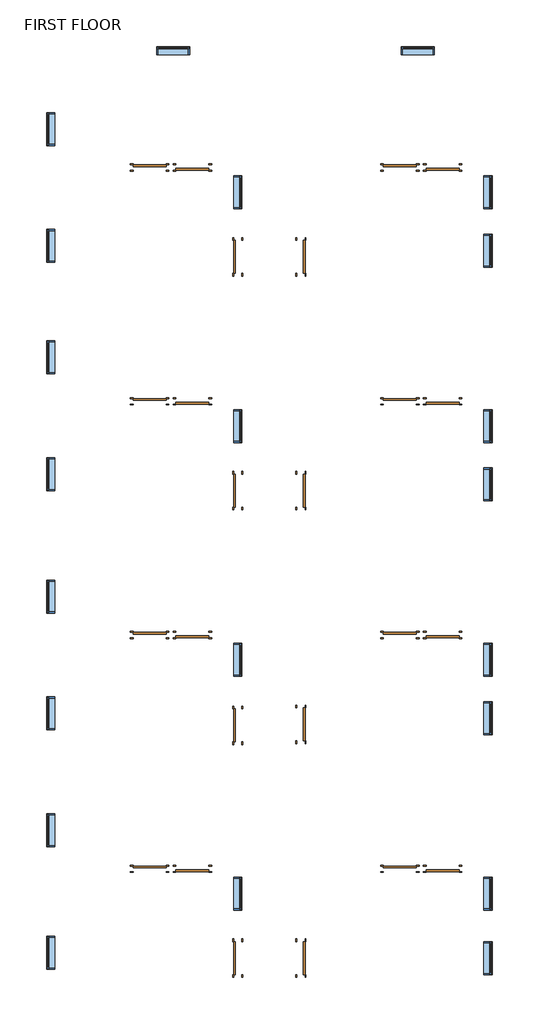
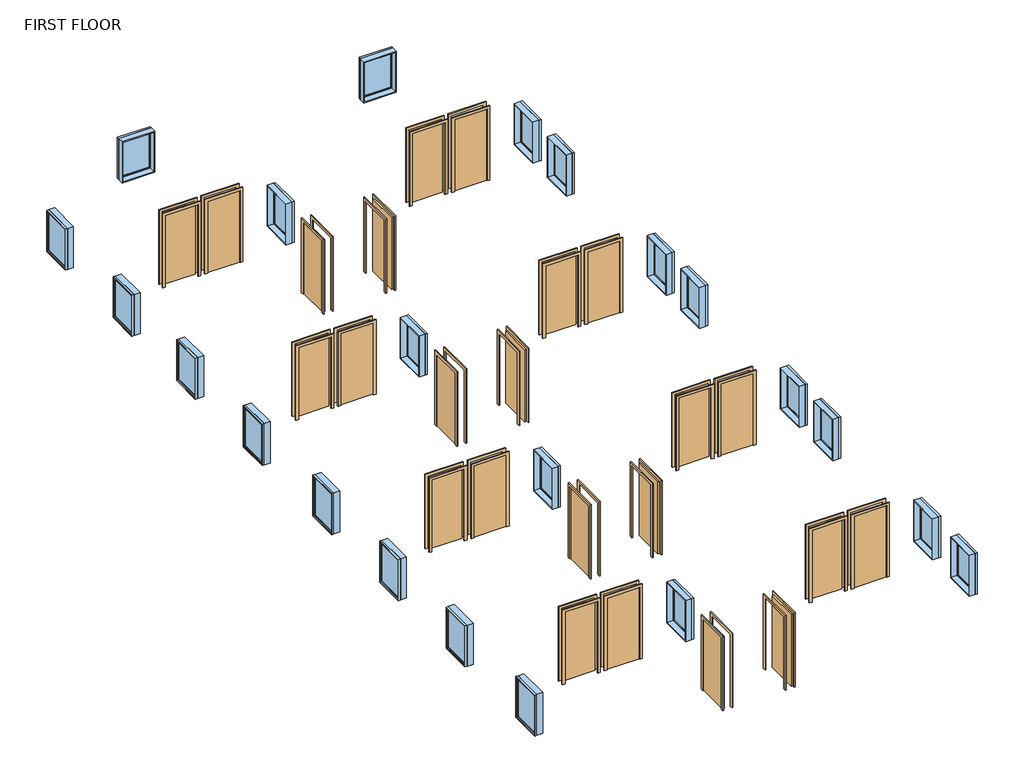
# One storey: 24 doors, 22 windows.
"""IFC4 building model written with IfcOpenShell, lengths in millimetres."""

from ifc_helpers import new_model, si_unit, origin, place, context, project, spatial, transform, mapped, element, save
from components import door_686f89d2, door_16372e1c, door_a90ba1ad, door_0ca8825f, window_c1f32544

model = new_model("IFC4")

# Units and contexts
model_context = context("Model", 3, world=origin())
ifc_project = project(units=[si_unit("LENGTHUNIT", "METRE", prefix="MILLI")], contexts=[model_context])

# Site, building, storey
site = spatial("IfcSite", under=ifc_project)
building = spatial("IfcBuilding", under=site)
storey = spatial("IfcBuildingStorey", under=building, Name="FIRST FLOOR", Elevation=3200.4)

# Doors
placement = place(None, origin())
door_shape = door_686f89d2(model_context)
element("IfcDoor", 1, ObjectType="Single-Flush : 36\" x 84\"", at=placement, inside=storey, context=model_context, shape_type="MappedRepresentation", body=[
    mapped(door_shape, transform((-9863.5902461, 11952.2710592, 3200.4), x_axis=(-1.0, 0.0, 0.0), y_axis=(0.0, -1.0, 0.0), z_axis=(0.0, 0.0, 1.0))),
])
element("IfcDoor", 2, ObjectType="Single-Flush : 36\" x 84\"", at=placement, inside=storey, context=model_context, shape_type="MappedRepresentation", body=[
    mapped(door_shape, transform((-2929.3902461, -7478.7289408, 3200.4), x_axis=(-1.0, 0.0, 0.0), y_axis=(0.0, -1.0, 0.0), z_axis=(0.0, 0.0, 1.0))),
])
element("IfcDoor", 3, ObjectType="Single-Flush : 36\" x 84\"", at=placement, inside=storey, context=model_context, shape_type="MappedRepresentation", body=[
    mapped(door_shape, transform((-2929.3902461, 11952.2710592, 3200.4), x_axis=(-1.0, 0.0, 0.0), y_axis=(0.0, -1.0, 0.0), z_axis=(0.0, 0.0, 1.0))),
])
element("IfcDoor", 4, ObjectType="Single-Flush : 36\" x 84\"", at=placement, inside=storey, context=model_context, shape_type="MappedRepresentation", body=[
    mapped(door_shape, transform((-2929.3902461, 5475.2710592, 3200.4), x_axis=(-1.0, 0.0, 0.0), y_axis=(0.0, -1.0, 0.0), z_axis=(0.0, 0.0, 1.0))),
])
element("IfcDoor", 5, ObjectType="Single-Flush : 36\" x 84\"", at=placement, inside=storey, context=model_context, shape_type="MappedRepresentation", body=[
    mapped(door_shape, transform((-2929.3902461, -1001.7289408, 3200.4), x_axis=(-1.0, 0.0, 0.0), y_axis=(0.0, -1.0, 0.0), z_axis=(0.0, 0.0, 1.0))),
])
element("IfcDoor", 6, ObjectType="Single-Flush : 36\" x 84\"", at=placement, inside=storey, context=model_context, shape_type="MappedRepresentation", body=[
    mapped(door_shape, transform((-9863.5902461, -7478.7289408, 3200.4), x_axis=(-1.0, 0.0, 0.0), y_axis=(0.0, -1.0, 0.0), z_axis=(0.0, 0.0, 1.0))),
])
element("IfcDoor", 7, ObjectType="Single-Flush : 36\" x 84\"", at=placement, inside=storey, context=model_context, shape_type="MappedRepresentation", body=[
    mapped(door_shape, transform((-9863.5902461, -1001.7289408, 3200.4), x_axis=(-1.0, 0.0, 0.0), y_axis=(0.0, -1.0, 0.0), z_axis=(0.0, 0.0, 1.0))),
])
element("IfcDoor", 8, ObjectType="Single-Flush : 36\" x 84\"", at=placement, inside=storey, context=model_context, shape_type="MappedRepresentation", body=[
    mapped(door_shape, transform((-9863.5902461, 5475.2710592, 3200.4), x_axis=(-1.0, 0.0, 0.0), y_axis=(0.0, -1.0, 0.0), z_axis=(0.0, 0.0, 1.0))),
])
door_2_shape = door_16372e1c(model_context)
element("IfcDoor", 9, ObjectType="Single-Flush : 36\" x 84\"", at=placement, inside=storey, context=model_context, shape_type="MappedRepresentation", body=[
    mapped(door_2_shape, transform((-8682.4902461, 11952.2710592, 3200.4), x_axis=(-1.0, 0.0, 0.0), y_axis=(0.0, -1.0, 0.0), z_axis=(0.0, 0.0, 1.0))),
])
element("IfcDoor", 10, ObjectType="Single-Flush : 36\" x 84\"", at=placement, inside=storey, context=model_context, shape_type="MappedRepresentation", body=[
    mapped(door_2_shape, transform((-1748.2902461, -7478.7289408, 3200.4), x_axis=(-1.0, 0.0, 0.0), y_axis=(0.0, -1.0, 0.0), z_axis=(0.0, 0.0, 1.0))),
])
element("IfcDoor", 11, ObjectType="Single-Flush : 36\" x 84\"", at=placement, inside=storey, context=model_context, shape_type="MappedRepresentation", body=[
    mapped(door_2_shape, transform((-1748.2902461, -1001.7289408, 3200.4), x_axis=(-1.0, 0.0, 0.0), y_axis=(0.0, -1.0, 0.0), z_axis=(0.0, 0.0, 1.0))),
])
element("IfcDoor", 12, ObjectType="Single-Flush : 36\" x 84\"", at=placement, inside=storey, context=model_context, shape_type="MappedRepresentation", body=[
    mapped(door_2_shape, transform((-1748.2902461, 5475.2710592, 3200.4), x_axis=(-1.0, 0.0, 0.0), y_axis=(0.0, -1.0, 0.0), z_axis=(0.0, 0.0, 1.0))),
])
element("IfcDoor", 13, ObjectType="Single-Flush : 36\" x 84\"", at=placement, inside=storey, context=model_context, shape_type="MappedRepresentation", body=[
    mapped(door_2_shape, transform((-1748.2902461, 11952.2710592, 3200.4), x_axis=(-1.0, 0.0, 0.0), y_axis=(0.0, -1.0, 0.0), z_axis=(0.0, 0.0, 1.0))),
])
element("IfcDoor", 14, ObjectType="Single-Flush : 36\" x 84\"", at=placement, inside=storey, context=model_context, shape_type="MappedRepresentation", body=[
    mapped(door_2_shape, transform((-8682.4902461, -7478.7289408, 3200.4), x_axis=(-1.0, 0.0, 0.0), y_axis=(0.0, -1.0, 0.0), z_axis=(0.0, 0.0, 1.0))),
])
element("IfcDoor", 15, ObjectType="Single-Flush : 36\" x 84\"", at=placement, inside=storey, context=model_context, shape_type="MappedRepresentation", body=[
    mapped(door_2_shape, transform((-8682.4902461, -1001.7289408, 3200.4), x_axis=(-1.0, 0.0, 0.0), y_axis=(0.0, -1.0, 0.0), z_axis=(0.0, 0.0, 1.0))),
])
element("IfcDoor", 16, ObjectType="Single-Flush : 36\" x 84\"", at=placement, inside=storey, context=model_context, shape_type="MappedRepresentation", body=[
    mapped(door_2_shape, transform((-8682.4902461, 5475.2710592, 3200.4), x_axis=(-1.0, 0.0, 0.0), y_axis=(0.0, -1.0, 0.0), z_axis=(0.0, 0.0, 1.0))),
])
door_3_shape = door_a90ba1ad(model_context)
element("IfcDoor", 17, ObjectType="Single-Flush : 36\" x 84\"", at=placement, inside=storey, context=model_context, shape_type="MappedRepresentation", body=[
    mapped(door_3_shape, transform((-7425.1902461, 9475.7710592, 3200.4), x_axis=(0.0, -1.0, 0.0), y_axis=(1.0, 0.0, 0.0), z_axis=(0.0, 0.0, 1.0))),
])
element("IfcDoor", 18, ObjectType="Single-Flush : 36\" x 84\"", at=placement, inside=storey, context=model_context, shape_type="MappedRepresentation", body=[
    mapped(door_3_shape, transform((-7425.1902461, 2998.7710592, 3200.4), x_axis=(0.0, -1.0, 0.0), y_axis=(1.0, 0.0, 0.0), z_axis=(0.0, 0.0, 1.0))),
])
element("IfcDoor", 19, ObjectType="Single-Flush : 36\" x 84\"", at=placement, inside=storey, context=model_context, shape_type="MappedRepresentation", body=[
    mapped(door_3_shape, transform((-7425.1902461, -3503.6289408, 3200.4), x_axis=(0.0, -1.0, 0.0), y_axis=(1.0, 0.0, 0.0), z_axis=(0.0, 0.0, 1.0))),
])
element("IfcDoor", 20, ObjectType="Single-Flush : 36\" x 84\"", at=placement, inside=storey, context=model_context, shape_type="MappedRepresentation", body=[
    mapped(door_3_shape, transform((-7425.1902461, -9955.2289408, 3200.4), x_axis=(0.0, -1.0, 0.0), y_axis=(1.0, 0.0, 0.0), z_axis=(0.0, 0.0, 1.0))),
])
door_4_shape = door_0ca8825f(model_context)
element("IfcDoor", 21, ObjectType="Single-Flush : 36\" x 84\"", at=placement, inside=storey, context=model_context, shape_type="MappedRepresentation", body=[
    mapped(door_4_shape, transform((-5672.5902461, 9475.7710592, 3200.4), x_axis=(0.0, -1.0, 0.0), y_axis=(1.0, 0.0, 0.0), z_axis=(0.0, 0.0, 1.0))),
])
element("IfcDoor", 22, ObjectType="Single-Flush : 36\" x 84\"", at=placement, inside=storey, context=model_context, shape_type="MappedRepresentation", body=[
    mapped(door_4_shape, transform((-5672.5902461, 2998.7710592, 3200.4), x_axis=(0.0, -1.0, 0.0), y_axis=(1.0, 0.0, 0.0), z_axis=(0.0, 0.0, 1.0))),
])
element("IfcDoor", 23, ObjectType="Single-Flush : 36\" x 84\"", at=placement, inside=storey, context=model_context, shape_type="MappedRepresentation", body=[
    mapped(door_4_shape, transform((-5672.5902461, -3478.2289408, 3200.4), x_axis=(0.0, -1.0, 0.0), y_axis=(1.0, 0.0, 0.0), z_axis=(0.0, 0.0, 1.0))),
])
element("IfcDoor", 24, ObjectType="Single-Flush : 36\" x 84\"", at=placement, inside=storey, context=model_context, shape_type="MappedRepresentation", body=[
    mapped(door_4_shape, transform((-5672.5902461, -9955.2289408, 3200.4), x_axis=(0.0, -1.0, 0.0), y_axis=(1.0, 0.0, 0.0), z_axis=(0.0, 0.0, 1.0))),
])

# Windows
window_shape = window_c1f32544(model_context)
element("IfcWindow", 25, ObjectType="Fixed : 36\" x 48\"", at=placement, inside=storey, context=model_context, shape_type="MappedRepresentation", body=[
    mapped(window_shape, transform((-7425.1902461, 4751.3710592, 3200.4), x_axis=(0.0, -1.0, 0.0), y_axis=(1.0, 0.0, 0.0), z_axis=(0.0, 0.0, 1.0))),
])
element("IfcWindow", 26, ObjectType="Fixed : 36\" x 48\"", at=placement, inside=storey, context=model_context, shape_type="MappedRepresentation", body=[
    mapped(window_shape, transform((-7425.1902461, -1725.6289408, 3200.4), x_axis=(0.0, -1.0, 0.0), y_axis=(1.0, 0.0, 0.0), z_axis=(0.0, 0.0, 1.0))),
])
element("IfcWindow", 27, ObjectType="Fixed : 36\" x 48\"", at=placement, inside=storey, context=model_context, shape_type="MappedRepresentation", body=[
    mapped(window_shape, transform((-7425.1902461, -8202.6289408, 3200.4), x_axis=(0.0, -1.0, 0.0), y_axis=(1.0, 0.0, 0.0), z_axis=(0.0, 0.0, 1.0))),
])
element("IfcWindow", 28, ObjectType="Fixed : 36\" x 48\"", at=placement, inside=storey, context=model_context, shape_type="MappedRepresentation", body=[
    mapped(window_shape, transform((-7425.1902461, 11228.3710592, 3200.4), x_axis=(0.0, -1.0, 0.0), y_axis=(1.0, 0.0, 0.0), z_axis=(0.0, 0.0, 1.0))),
])
element("IfcWindow", 29, ObjectType="Fixed : 36\" x 48\"", at=placement, inside=storey, context=model_context, shape_type="MappedRepresentation", body=[
    mapped(window_shape, transform((-490.9902461, 11228.3710592, 3200.4), x_axis=(0.0, -1.0, 0.0), y_axis=(1.0, 0.0, 0.0), z_axis=(0.0, 0.0, 1.0))),
])
element("IfcWindow", 30, ObjectType="Fixed : 36\" x 48\"", at=placement, inside=storey, context=model_context, shape_type="MappedRepresentation", body=[
    mapped(window_shape, transform((-490.9902461, 9609.1210592, 3200.4), x_axis=(0.0, -1.0, 0.0), y_axis=(1.0, 0.0, 0.0), z_axis=(0.0, 0.0, 1.0))),
])
element("IfcWindow", 31, ObjectType="Fixed : 36\" x 48\"", at=placement, inside=storey, context=model_context, shape_type="MappedRepresentation", body=[
    mapped(window_shape, transform((-490.9902461, 4751.3710592, 3200.4), x_axis=(0.0, -1.0, 0.0), y_axis=(1.0, 0.0, 0.0), z_axis=(0.0, 0.0, 1.0))),
])
element("IfcWindow", 32, ObjectType="Fixed : 36\" x 48\"", at=placement, inside=storey, context=model_context, shape_type="MappedRepresentation", body=[
    mapped(window_shape, transform((-490.9902461, 3132.1210592, 3200.4), x_axis=(0.0, -1.0, 0.0), y_axis=(1.0, 0.0, 0.0), z_axis=(0.0, 0.0, 1.0))),
])
element("IfcWindow", 33, ObjectType="Fixed : 36\" x 48\"", at=placement, inside=storey, context=model_context, shape_type="MappedRepresentation", body=[
    mapped(window_shape, transform((-490.9902461, -1725.6289408, 3200.4), x_axis=(0.0, -1.0, 0.0), y_axis=(1.0, 0.0, 0.0), z_axis=(0.0, 0.0, 1.0))),
])
element("IfcWindow", 34, ObjectType="Fixed : 36\" x 48\"", at=placement, inside=storey, context=model_context, shape_type="MappedRepresentation", body=[
    mapped(window_shape, transform((-490.9902461, -3344.8789408, 3200.4), x_axis=(0.0, -1.0, 0.0), y_axis=(1.0, 0.0, 0.0), z_axis=(0.0, 0.0, 1.0))),
])
element("IfcWindow", 35, ObjectType="Fixed : 36\" x 48\"", at=placement, inside=storey, context=model_context, shape_type="MappedRepresentation", body=[
    mapped(window_shape, transform((-490.9902461, -8202.6289408, 3200.4), x_axis=(0.0, -1.0, 0.0), y_axis=(1.0, 0.0, 0.0), z_axis=(0.0, 0.0, 1.0))),
])
element("IfcWindow", 36, ObjectType="Fixed : 36\" x 48\"", at=placement, inside=storey, context=model_context, shape_type="MappedRepresentation", body=[
    mapped(window_shape, transform((-490.9902461, -9993.3289408, 3200.4), x_axis=(0.0, -1.0, 0.0), y_axis=(1.0, 0.0, 0.0), z_axis=(0.0, 0.0, 1.0))),
])
element("IfcWindow", 37, ObjectType="Fixed : 36\" x 48\"", at=placement, inside=storey, context=model_context, shape_type="MappedRepresentation", body=[
    mapped(window_shape, transform((-2395.9902461, 15190.7710592, 3200.4), x_axis=(1.0, 0.0, 0.0), y_axis=(0.0, 1.0, 0.0), z_axis=(0.0, 0.0, 1.0))),
])
element("IfcWindow", 38, ObjectType="Fixed : 36\" x 48\"", at=placement, inside=storey, context=model_context, shape_type="MappedRepresentation", body=[
    mapped(window_shape, transform((-9177.7902461, 15190.7710592, 3200.4), x_axis=(1.0, 0.0, 0.0), y_axis=(0.0, 1.0, 0.0), z_axis=(0.0, 0.0, 1.0))),
])
element("IfcWindow", 39, ObjectType="Fixed : 36\" x 48\"", at=placement, inside=storey, context=model_context, shape_type="MappedRepresentation", body=[
    mapped(window_shape, transform((-12606.7902461, 13057.1710592, 3200.4), x_axis=(0.0, 1.0, 0.0), y_axis=(-1.0, 0.0, 0.0), z_axis=(0.0, 0.0, 1.0))),
])
element("IfcWindow", 40, ObjectType="Fixed : 36\" x 48\"", at=placement, inside=storey, context=model_context, shape_type="MappedRepresentation", body=[
    mapped(window_shape, transform((-12606.7902461, 9818.6710592, 3200.4), x_axis=(0.0, 1.0, 0.0), y_axis=(-1.0, 0.0, 0.0), z_axis=(0.0, 0.0, 1.0))),
])
element("IfcWindow", 41, ObjectType="Fixed : 36\" x 48\"", at=placement, inside=storey, context=model_context, shape_type="MappedRepresentation", body=[
    mapped(window_shape, transform((-12606.7902461, 6732.5710592, 3200.4), x_axis=(0.0, 1.0, 0.0), y_axis=(-1.0, 0.0, 0.0), z_axis=(0.0, 0.0, 1.0))),
])
element("IfcWindow", 42, ObjectType="Fixed : 36\" x 48\"", at=placement, inside=storey, context=model_context, shape_type="MappedRepresentation", body=[
    mapped(window_shape, transform((-12606.7902461, 3494.0710592, 3200.4), x_axis=(0.0, 1.0, 0.0), y_axis=(-1.0, 0.0, 0.0), z_axis=(0.0, 0.0, 1.0))),
])
element("IfcWindow", 43, ObjectType="Fixed : 36\" x 48\"", at=placement, inside=storey, context=model_context, shape_type="MappedRepresentation", body=[
    mapped(window_shape, transform((-12606.7902461, 103.1710592, 3200.4), x_axis=(0.0, 1.0, 0.0), y_axis=(-1.0, 0.0, 0.0), z_axis=(0.0, 0.0, 1.0))),
])
element("IfcWindow", 44, ObjectType="Fixed : 36\" x 48\"", at=placement, inside=storey, context=model_context, shape_type="MappedRepresentation", body=[
    mapped(window_shape, transform((-12606.7902461, -3135.3289408, 3200.4), x_axis=(0.0, 1.0, 0.0), y_axis=(-1.0, 0.0, 0.0), z_axis=(0.0, 0.0, 1.0))),
])
element("IfcWindow", 45, ObjectType="Fixed : 36\" x 48\"", at=placement, inside=storey, context=model_context, shape_type="MappedRepresentation", body=[
    mapped(window_shape, transform((-12606.7902461, -6373.8289408, 3200.4), x_axis=(0.0, 1.0, 0.0), y_axis=(-1.0, 0.0, 0.0), z_axis=(0.0, 0.0, 1.0))),
])
element("IfcWindow", 46, ObjectType="Fixed : 36\" x 48\"", at=placement, inside=storey, context=model_context, shape_type="MappedRepresentation", body=[
    mapped(window_shape, transform((-12606.7902461, -9764.7289408, 3200.4), x_axis=(0.0, 1.0, 0.0), y_axis=(-1.0, 0.0, 0.0), z_axis=(0.0, 0.0, 1.0))),
])

save(model, "model.ifc")

# Revit data of these elements
# Type "Single-Flush : 36\" x 84\""
#   Type Mark = "1"
#   Construction Type Id = "MDOOR"
#   Assembly Code = "C1020"
#   Analytic Construction = "Metal"
#   Thickness = 0' - 2"
#   Heat Transfer Coefficient (U) = 0.651978 BTU/(h·ft²·°F)
#   Height = 7' - 0"
#   Trim Projection Ext = 0' - 1"
#   Trim Projection Int = 0' - 1"
#   Trim Width = 0' - 3"
#   Width = 3' - 0"
#   Define Thermal Properties by = 1
#   Door Material = Door - Panel
#   Frame Material = Door - Frame
#   Visual Light Transmittance = 0
#   Solar Heat Gain Coefficient = 0
#   Function = (empty or 0)
#   Wall Closure = (empty or 0)
# Type "Fixed : 36\" x 48\""
#   Type Mark = "1"
#   Construction Type Id = "GSP4R"
#   Assembly Code = "B2020100"
#   Analytic Construction = "1/8 in Pilkington single glazing"
#   Visual Light Transmittance = 0.9
#   Solar Heat Gain Coefficient = 0.78
#   Heat Transfer Coefficient (U) = 0.6496 BTU/(h·ft²·°F)
#   Height = 4' - 0"
#   Default Sill Height = 3' - 0"
#   Width = 3' - 0"
#   Window Inset = 0' - 0 3/4"
#   Define Thermal Properties by = 1
#   Glass Pane Material = Glass
#   Sash Material = Sash
#   Wall Closure = (empty or 0)
# Elements 1, 2, 3, 4, 5, 6, 7, 8, 9, 10, 11, 12, 13, 14, 15, 16, 17, 18, 19, 20, 21, 22, 23, 24 (IfcDoor, "Single-Flush : 36\" x 84\"")
#   Phase Created = New Construction
#   Materials on its faces: "Door - Frame", "Door - Panel"
# Element 25 (IfcWindow, "Fixed : 36\" x 48\"")
#   Mark = "27"
#   Phase Created = New Construction
#   Materials on its faces: "Sash", "Glass"
# Element 26 (IfcWindow, "Fixed : 36\" x 48\"")
#   Mark = "28"
#   Phase Created = New Construction
#   Materials on its faces: "Sash", "Glass"
# Element 27 (IfcWindow, "Fixed : 36\" x 48\"")
#   Mark = "29"
#   Phase Created = New Construction
#   Materials on its faces: "Sash", "Glass"
# Element 28 (IfcWindow, "Fixed : 36\" x 48\"")
#   Mark = "30"
#   Phase Created = New Construction
#   Materials on its faces: "Sash", "Glass"
# Element 29 (IfcWindow, "Fixed : 36\" x 48\"")
#   Mark = "31"
#   Phase Created = New Construction
#   Materials on its faces: "Sash", "Glass"
# Element 30 (IfcWindow, "Fixed : 36\" x 48\"")
#   Mark = "32"
#   Phase Created = New Construction
#   Materials on its faces: "Sash", "Glass"
# Element 31 (IfcWindow, "Fixed : 36\" x 48\"")
#   Mark = "33"
#   Phase Created = New Construction
#   Materials on its faces: "Sash", "Glass"
# Element 32 (IfcWindow, "Fixed : 36\" x 48\"")
#   Mark = "34"
#   Phase Created = New Construction
#   Materials on its faces: "Sash", "Glass"
# Element 33 (IfcWindow, "Fixed : 36\" x 48\"")
#   Mark = "35"
#   Phase Created = New Construction
#   Materials on its faces: "Sash", "Glass"
# Element 34 (IfcWindow, "Fixed : 36\" x 48\"")
#   Mark = "36"
#   Phase Created = New Construction
#   Materials on its faces: "Sash", "Glass"
# Element 35 (IfcWindow, "Fixed : 36\" x 48\"")
#   Mark = "37"
#   Phase Created = New Construction
#   Materials on its faces: "Sash", "Glass"
# Element 36 (IfcWindow, "Fixed : 36\" x 48\"")
#   Mark = "38"
#   Phase Created = New Construction
#   Materials on its faces: "Sash", "Glass"
# Element 37 (IfcWindow, "Fixed : 36\" x 48\"")
#   Mark = "39"
#   Phase Created = New Construction
#   Materials on its faces: "Sash", "Glass"
# Element 38 (IfcWindow, "Fixed : 36\" x 48\"")
#   Mark = "40"
#   Phase Created = New Construction
#   Materials on its faces: "Sash", "Glass"
# Element 39 (IfcWindow, "Fixed : 36\" x 48\"")
#   Mark = "41"
#   Phase Created = New Construction
#   Materials on its faces: "Sash", "Glass"
# Element 40 (IfcWindow, "Fixed : 36\" x 48\"")
#   Mark = "42"
#   Phase Created = New Construction
#   Materials on its faces: "Sash", "Glass"
# Element 41 (IfcWindow, "Fixed : 36\" x 48\"")
#   Mark = "43"
#   Phase Created = New Construction
#   Materials on its faces: "Sash", "Glass"
# Element 42 (IfcWindow, "Fixed : 36\" x 48\"")
#   Mark = "44"
#   Phase Created = New Construction
#   Materials on its faces: "Sash", "Glass"
# Element 43 (IfcWindow, "Fixed : 36\" x 48\"")
#   Mark = "45"
#   Phase Created = New Construction
#   Materials on its faces: "Sash", "Glass"
# Element 44 (IfcWindow, "Fixed : 36\" x 48\"")
#   Mark = "46"
#   Phase Created = New Construction
#   Materials on its faces: "Sash", "Glass"
# Element 45 (IfcWindow, "Fixed : 36\" x 48\"")
#   Mark = "47"
#   Phase Created = New Construction
#   Materials on its faces: "Sash", "Glass"
# Element 46 (IfcWindow, "Fixed : 36\" x 48\"")
#   Mark = "48"
#   Phase Created = New Construction
#   Materials on its faces: "Sash", "Glass"
# Materials
#   "Door - Panel": class "Wood", colour RGB 210 159 95, transparency 0
#   "Door - Frame": colour RGB 118 70 51, transparency 0
#   "Glass": class "Glass", colour RGB 0 128 192, transparency 0.75, Description = "Soda Lime Glass", Cost = 0
#   "Sash": class "Wood", colour RGB 224 178 126, transparency 0
